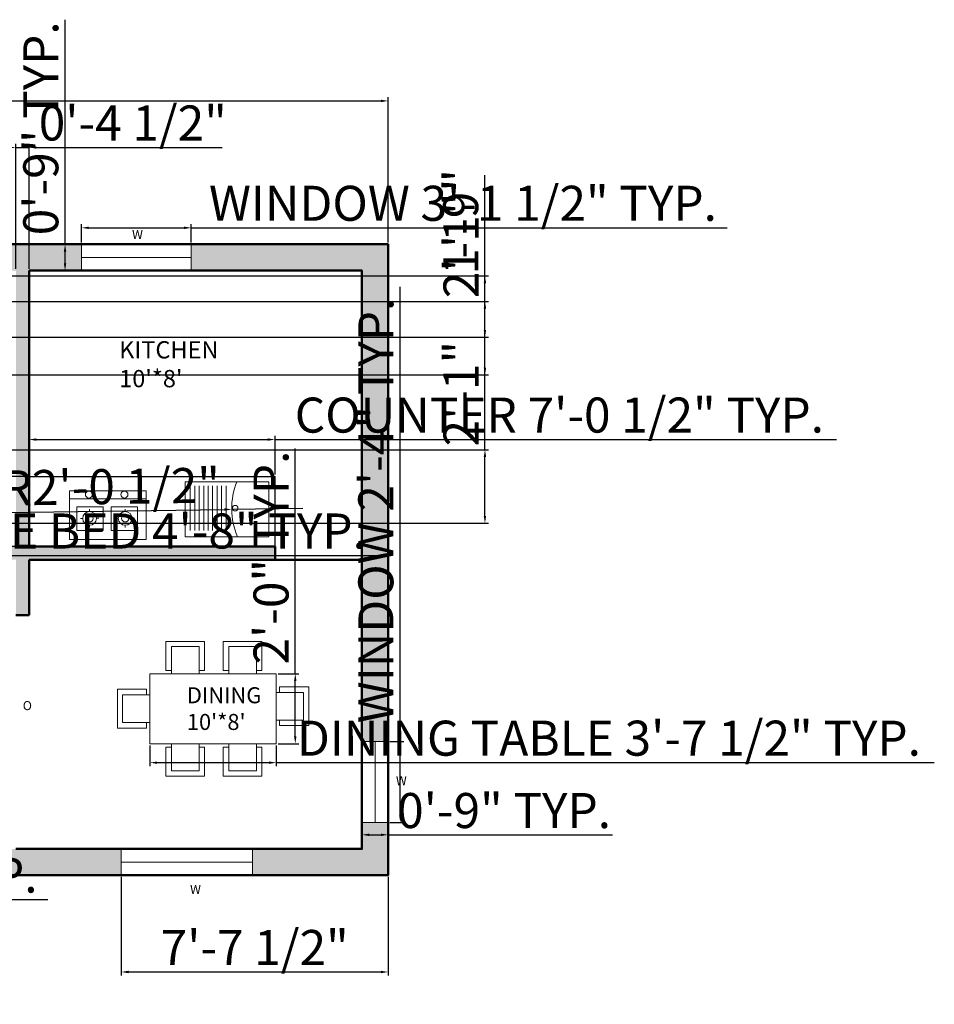
# Model space of a CAD drawing. Units: inches. Extents: x 2225 to 3094, y 1739 to 2599.
# Tile 4 of 5: x 2780 to 3094, y 1755 to 2092. Entities that reach past the tile are written whole.
import ezdxf

# ---------------------------------------------------------------- set-up
doc = ezdxf.new("R2010")
doc.units = ezdxf.units.IN
for name, color, linetype, lineweight in [('A-ANNO-DIMS', 2, 'Continuous', 18), ('A-ANNO-TEXT', 7, 'Continuous', 18), ('A-AREA-IDEN', 7, 'Continuous', 18), ('A-EQPM', 8, 'Continuous', 18), ('A-FLOR-CASE', 9, 'Continuous', 25), ('A-FLOR-FIXT', 9, 'Continuous', 18), ('A-FURN', 8, 'Continuous', 18), ('A-WALL-PATT', 160, 'Continuous', 13), ('WALL', 7, 'Continuous', 50), ('WINDOW', 130, 'Continuous', 18)]:
    doc.layers.add(name, color=color, linetype=linetype, lineweight=lineweight)
doc.styles.get("Standard").update_dxf_attribs({"font": 'arial.ttf'})
doc.dimstyles.new('ISO-25', dxfattribs={"dimtxt": 12, "dimasz": 2.5, "dimexe": 1.25, "dimexo": 0.625, "dimtad": 1, "dimdec": 0, "dimlunit": 4, "dimtxsty": 'Standard', "dimcen": 2.5, "dimadec": 0, "dimazin": 0, "dimtfac": 1, "dimtdec": 0, "dimtmove": 0, "dimatfit": 3, "dimfxl": 1, "dimarcsym": 0})

# ---------------------------------------------------------------- blocks, each defined once
blk = doc.blocks.new('*D7')
at = {"layer": 'A-ANNO-DIMS', "color": 0, "lineweight": -2, "transparency": 16777216}
for p, q in [((2282.56, 2016.04), (2282.56, 2065.75)), ((2285.06, 2064.5), (2904.06, 2064.5)), ((2906.56, 2016.04), (2906.56, 2065.75))]:
    blk.add_line(p, q, dxfattribs=at)
at = {"layer": 'A-ANNO-DIMS', "color": 0, "transparency": 16777216}
for points in [[(2285.06, 2064.92), (2285.06, 2064.08), (2282.56, 2064.5)], [(2904.06, 2064.92), (2904.06, 2064.08), (2906.56, 2064.5)]]:
    blk.add_solid(points, dxfattribs=at)
at = {"layer": 'Defpoints', "color": 0, "transparency": 16777216}
for p in [(2906.56, 2064.5), (2282.56, 2015.41), (2906.56, 2015.41)]:
    blk.add_point(p, dxfattribs=at)
at = {"layer": 'A-ANNO-DIMS', "color": 0, "transparency": 16777216, "insert": (2594.56, 2071.25), "char_height": 12, "attachment_point": 5}
blk.add_mtext("52'", dxfattribs=at)
blk = doc.blocks.new('CHAIR-DINING')
for p, q in [((0, 1.13), (0, 11.11)), ((0, 11.11), (13.29, 11.11)), ((13.29, 1.13), (13.29, 11.11)), ((1.95, 1.13), (0, 1.13)), ((13.29, 1.13), (11.43, 1.13))]:
    blk.add_line(p, q)
blk.add_lwpolyline([(1.95, 0), (11.43, 0), (11.43, 9.33), (1.95, 9.33)], close=True)
blk = doc.blocks.new('TABLE-DINING')
blk.add_lwpolyline([(0, 23.93), (43.3, 23.93), (43.3, 0), (0, 0)], close=True)
blk = doc.blocks.new('COOKTOP-TWO-BURNER')
for p, q in [((0, 13.93), (26.27, 13.93)), ((6.81, 9.56), (6.81, 10.38)), ((19.02, 9.56), (19.02, 10.38)), ((4.52, 7.14), (3.73, 7.14)), ((9.26, 7.23), (10.04, 7.23)), ((16.73, 7.14), (15.94, 7.14)), ((21.47, 7.23), (22.24, 7.23)), ((6.9, 4.82), (6.9, 4.11)), ((19.11, 4.82), (19.11, 4.11))]:
    blk.add_line(p, q)
for points in [[(0, 0), (26.27, 0), (26.27, 16.66), (0, 16.66)], [(2.47, 11.19), (11.48, 11.19), (11.48, 3.09), (2.47, 3.09)], [(14.27, 11.19), (23.28, 11.19), (23.28, 3.09), (14.27, 3.09)]]:
    blk.add_lwpolyline(points, close=True)
for centre, radius in [((6.64, 15.37), 1.2), ((18.83, 15.37), 1.2), ((6.89, 7.19), 2.37), ((6.89, 7.19), 1.23), ((19.1, 7.19), 2.37), ((19.1, 7.19), 1.23)]:
    blk.add_circle(centre, radius)
blk = doc.blocks.new('SINK-DRAINBOARD')
for p, q in [((1.79, 17.4), (1.79, 2.15)), ((3.32, 17.4), (3.32, 2.15)), ((4.85, 17.4), (4.85, 2.15)), ((6.38, 17.4), (6.38, 2.15)), ((7.91, 17.4), (7.91, 2.15)), ((9.44, 17.4), (9.44, 2.15)), ((10.98, 17.4), (10.98, 2.15)), ((12.51, 17.4), (12.51, 2.15)), ((14.04, 17.4), (14.04, 2.15))]:
    blk.add_line(p, q)
blk.add_lwpolyline([(0, 0), (28.72, 0), (28.72, 18.77), (0, 18.77)], close=True)
blk.add_circle((17.16, 9.78), 0.951)
blk.add_arc((40.38, 9.7), 24.39, 158.1829, 203.4296)
blk = doc.blocks.new('WIN-37P6IN')
blk.add_line((0, 4.5), (37.6, 4.5))
blk.add_lwpolyline([(37.6, 0), (0, 0), (0, 9), (37.6, 9)], close=True)
blk = doc.blocks.new('WIN-44P9IN')
blk.add_line((0, 4.5), (44.94, 4.5))
blk.add_lwpolyline([(0, 0), (44.94, 0), (44.94, 9), (0, 9)], close=True)
blk = doc.blocks.new('WIN-27P8IN')
blk.add_line((4.5, 0), (4.5, 27.82))
blk.add_lwpolyline([(0, 0), (9, 0), (9, 27.82), (0, 27.82)], close=True)
blk = doc.blocks.new('KITCHEN-COUNTER-RUN')
for p, q in [((0, 0), (0, 24)), ((0, 24), (84.25, 24)), ((84.25, 0), (84.25, 24))]:
    blk.add_line(p, q)
blk = doc.blocks.new('*D26')
at = {"layer": 'A-ANNO-DIMS', "color": 0, "lineweight": -2, "transparency": 16777216}
for p, q in [((2666.23, 1916.66), (2666.23, 1907.61)), ((2722.41, 1916.66), (2722.41, 1907.61)), ((2668.73, 1908.86), (2719.91, 1908.86)), ((2722.41, 1908.86), (2904.52, 1908.86))]:
    blk.add_line(p, q, dxfattribs=at)
at = {"layer": 'A-ANNO-DIMS', "color": 0, "transparency": 16777216}
for points in [[(2668.73, 1909.27), (2668.73, 1908.44), (2666.23, 1908.86)], [(2719.91, 1909.27), (2719.91, 1908.44), (2722.41, 1908.86)]]:
    blk.add_solid(points, dxfattribs=at)
at = {"layer": 'Defpoints', "color": 0, "transparency": 16777216}
for p in [(2666.23, 1917.28), (2722.41, 1917.28), (2722.41, 1908.86)]:
    blk.add_point(p, dxfattribs=at)
at = {"layer": 'A-ANNO-DIMS', "color": 0, "transparency": 16777216, "insert": (2814.71, 1915.69), "char_height": 12, "attachment_point": 5}
blk.add_mtext('SINGLE BED 4\'-8" TYP.', dxfattribs=at)
blk = doc.blocks.new('*D30')
at = {"layer": 'A-ANNO-DIMS', "color": 0, "lineweight": -2, "transparency": 16777216}
for p, q in [((2824.95, 1843.8), (2824.95, 1836.68)), ((2868.25, 1843.8), (2868.25, 1836.68)), ((2827.45, 1837.93), (2865.75, 1837.93)), ((2868.25, 1837.93), (3093.61, 1837.93))]:
    blk.add_line(p, q, dxfattribs=at)
at = {"layer": 'A-ANNO-DIMS', "color": 0, "transparency": 16777216}
for points in [[(2827.45, 1838.34), (2827.45, 1837.51), (2824.95, 1837.93)], [(2865.75, 1838.34), (2865.75, 1837.51), (2868.25, 1837.93)]]:
    blk.add_solid(points, dxfattribs=at)
at = {"layer": 'Defpoints', "color": 0, "transparency": 16777216}
for p in [(2824.95, 1844.42), (2868.25, 1844.42), (2868.25, 1837.93)]:
    blk.add_point(p, dxfattribs=at)
at = {"layer": 'A-ANNO-DIMS', "color": 0, "transparency": 16777216, "insert": (2982.18, 1844.76), "char_height": 12, "attachment_point": 5}
blk.add_mtext('DINING TABLE 3\'-7 1/2" TYP.', dxfattribs=at)
blk = doc.blocks.new('*D31')
at = {"layer": 'A-ANNO-DIMS', "color": 0, "lineweight": -2, "transparency": 16777216}
for p, q in [((2874.75, 1868.35), (2874.75, 1945.46)), ((2868.88, 1868.35), (2876, 1868.35)), ((2874.75, 1846.92), (2874.75, 1865.85)), ((2868.88, 1844.42), (2876, 1844.42))]:
    blk.add_line(p, q, dxfattribs=at)
at = {"layer": 'A-ANNO-DIMS', "color": 0, "transparency": 16777216}
for points in [[(2874.33, 1865.85), (2875.17, 1865.85), (2874.75, 1868.35)], [(2874.33, 1846.92), (2875.17, 1846.92), (2874.75, 1844.42)]]:
    blk.add_solid(points, dxfattribs=at)
at = {"layer": 'Defpoints', "color": 0, "transparency": 16777216}
for p in [(2868.25, 1868.35), (2874.75, 1868.35), (2868.25, 1844.42)]:
    blk.add_point(p, dxfattribs=at)
at = {"layer": 'A-ANNO-DIMS', "color": 0, "transparency": 16777216, "insert": (2868, 1908.15), "char_height": 12, "attachment_point": 5, "rotation": 90}
blk.add_mtext('2\'-0" TYP.', dxfattribs=at)
blk = doc.blocks.new('*D42')
at = {"layer": 'A-ANNO-DIMS', "color": 0, "lineweight": -2, "transparency": 16777216}
for p, q in [((2783.56, 1936.54), (2783.56, 1949.8)), ((2786.06, 1948.55), (2865.31, 1948.55)), ((2867.81, 1936.54), (2867.81, 1949.8)), ((2867.81, 1948.55), (3060.07, 1948.55))]:
    blk.add_line(p, q, dxfattribs=at)
at = {"layer": 'A-ANNO-DIMS', "color": 0, "transparency": 16777216}
for points in [[(2786.06, 1948.97), (2786.06, 1948.13), (2783.56, 1948.55)], [(2865.31, 1948.97), (2865.31, 1948.13), (2867.81, 1948.55)]]:
    blk.add_solid(points, dxfattribs=at)
at = {"layer": 'Defpoints', "color": 0, "transparency": 16777216}
for p in [(2867.81, 1948.55), (2783.56, 1935.91), (2867.81, 1935.91)]:
    blk.add_point(p, dxfattribs=at)
at = {"layer": 'A-ANNO-DIMS', "color": 0, "transparency": 16777216, "insert": (2965.19, 1955.38), "char_height": 12, "attachment_point": 5}
blk.add_mtext('COUNTER 7\'-0 1/2" TYP.', dxfattribs=at)
blk = doc.blocks.new('*D43')
at = {"layer": 'A-ANNO-DIMS', "color": 0, "lineweight": -2, "transparency": 16777216}
for p, q in [((2770.92, 1935.91), (2770.92, 2013.01)), ((2782.93, 1935.91), (2769.67, 1935.91)), ((2770.92, 1914.41), (2770.92, 1933.41)), ((2782.93, 1911.91), (2769.67, 1911.91))]:
    blk.add_line(p, q, dxfattribs=at)
at = {"layer": 'A-ANNO-DIMS', "color": 0, "transparency": 16777216}
for points in [[(2770.5, 1933.41), (2771.34, 1933.41), (2770.92, 1935.91)], [(2770.5, 1914.41), (2771.34, 1914.41), (2770.92, 1911.91)]]:
    blk.add_solid(points, dxfattribs=at)
at = {"layer": 'Defpoints', "color": 0, "transparency": 16777216}
for p in [(2770.92, 1935.91), (2783.56, 1935.91), (2783.56, 1911.91)]:
    blk.add_point(p, dxfattribs=at)
at = {"layer": 'A-ANNO-DIMS', "color": 0, "transparency": 16777216, "insert": (2764.17, 1975.71), "char_height": 12, "attachment_point": 5, "rotation": 90}
blk.add_mtext('2\'-0" TYP.', dxfattribs=at)
blk = doc.blocks.new('*D46')
at = {"layer": 'A-ANNO-DIMS', "color": 0, "lineweight": -2, "transparency": 16777216}
for p, q in [((2801.54, 2016.04), (2801.54, 2022.3)), ((2804.04, 2021.05), (2836.64, 2021.05)), ((2839.14, 2016.04), (2839.14, 2022.3)), ((2839.14, 2021.05), (3022.7, 2021.05))]:
    blk.add_line(p, q, dxfattribs=at)
at = {"layer": 'A-ANNO-DIMS', "color": 0, "transparency": 16777216}
for points in [[(2804.04, 2021.47), (2804.04, 2020.63), (2801.54, 2021.05)], [(2836.64, 2021.47), (2836.64, 2020.63), (2839.14, 2021.05)]]:
    blk.add_solid(points, dxfattribs=at)
at = {"layer": 'Defpoints', "color": 0, "transparency": 16777216}
for p in [(2839.14, 2021.05), (2801.54, 2015.41), (2839.14, 2015.41)]:
    blk.add_point(p, dxfattribs=at)
at = {"layer": 'A-ANNO-DIMS', "color": 0, "transparency": 16777216, "insert": (2932.17, 2027.89), "char_height": 12, "attachment_point": 5}
blk.add_mtext('WINDOW 3\'-1 1/2" TYP.', dxfattribs=at)
blk = doc.blocks.new('*D47')
at = {"layer": 'A-ANNO-DIMS', "color": 0, "lineweight": -2, "transparency": 16777216}
for p, q in [((2795.9, 2015.41), (2795.9, 2092.31)), ((2800.91, 2015.41), (2794.65, 2015.41)), ((2795.9, 2008.91), (2795.9, 2012.91)), ((2800.91, 2006.41), (2794.65, 2006.41))]:
    blk.add_line(p, q, dxfattribs=at)
at = {"layer": 'A-ANNO-DIMS', "color": 0, "transparency": 16777216}
for points in [[(2795.48, 2012.91), (2796.32, 2012.91), (2795.9, 2015.41)], [(2795.48, 2008.91), (2796.32, 2008.91), (2795.9, 2006.41)]]:
    blk.add_solid(points, dxfattribs=at)
at = {"layer": 'Defpoints', "color": 0, "transparency": 16777216}
for p in [(2795.9, 2015.41), (2801.54, 2015.41), (2801.54, 2006.41)]:
    blk.add_point(p, dxfattribs=at)
at = {"layer": 'A-ANNO-DIMS', "color": 0, "transparency": 16777216, "insert": (2789.15, 2055.11), "char_height": 12, "attachment_point": 5, "rotation": 90}
blk.add_mtext('0\'-9" TYP.', dxfattribs=at)
blk = doc.blocks.new('*D50')
at = {"layer": 'A-ANNO-DIMS', "color": 0, "lineweight": -2, "transparency": 16777216}
for p, q in [((2910.73, 1845.22), (2910.73, 2000.82)), ((2907.18, 1845.22), (2911.98, 1845.22)), ((2910.73, 1819.9), (2910.73, 1842.72)), ((2907.18, 1817.4), (2911.98, 1817.4))]:
    blk.add_line(p, q, dxfattribs=at)
at = {"layer": 'A-ANNO-DIMS', "color": 0, "transparency": 16777216}
for points in [[(2910.31, 1842.72), (2911.15, 1842.72), (2910.73, 1845.22)], [(2910.31, 1819.9), (2911.15, 1819.9), (2910.73, 1817.4)]]:
    blk.add_solid(points, dxfattribs=at)
at = {"layer": 'Defpoints', "color": 0, "transparency": 16777216}
for p in [(2906.56, 1845.22), (2910.73, 1845.22), (2906.56, 1817.4)]:
    blk.add_point(p, dxfattribs=at)
at = {"layer": 'A-ANNO-DIMS', "color": 0, "transparency": 16777216, "insert": (2903.9, 1924.27), "char_height": 12, "attachment_point": 5, "rotation": 90}
blk.add_mtext('WINDOW 2\'-4" TYP.', dxfattribs=at)
blk = doc.blocks.new('*D51')
at = {"layer": 'A-ANNO-DIMS', "color": 0, "lineweight": -2, "transparency": 16777216}
for p, q in [((2897.56, 1816.77), (2897.56, 1811.98)), ((2906.56, 1816.77), (2906.56, 1811.98)), ((2900.06, 1813.23), (2904.06, 1813.23)), ((2906.56, 1813.23), (2983.45, 1813.23))]:
    blk.add_line(p, q, dxfattribs=at)
at = {"layer": 'A-ANNO-DIMS', "color": 0, "transparency": 16777216}
for points in [[(2900.06, 1813.64), (2900.06, 1812.81), (2897.56, 1813.23)], [(2904.06, 1813.64), (2904.06, 1812.81), (2906.56, 1813.23)]]:
    blk.add_solid(points, dxfattribs=at)
at = {"layer": 'Defpoints', "color": 0, "transparency": 16777216}
for p in [(2897.56, 1817.4), (2906.56, 1817.4), (2906.56, 1813.23)]:
    blk.add_point(p, dxfattribs=at)
at = {"layer": 'A-ANNO-DIMS', "color": 0, "transparency": 16777216, "insert": (2946.26, 1819.98), "char_height": 12, "attachment_point": 5}
blk.add_mtext('0\'-9" TYP.', dxfattribs=at)
blk = doc.blocks.new('*D52')
at = {"layer": 'A-ANNO-DIMS', "color": 0, "lineweight": -2, "transparency": 16777216}
for p, q in [((2550.8, 1798.79), (2550.8, 1789.81)), ((2606.48, 1798.79), (2606.48, 1789.81)), ((2553.3, 1791.06), (2603.98, 1791.06)), ((2606.48, 1791.06), (2790.04, 1791.06))]:
    blk.add_line(p, q, dxfattribs=at)
at = {"layer": 'A-ANNO-DIMS', "color": 0, "transparency": 16777216}
for points in [[(2553.3, 1791.48), (2553.3, 1790.64), (2550.8, 1791.06)], [(2603.98, 1791.48), (2603.98, 1790.64), (2606.48, 1791.06)]]:
    blk.add_solid(points, dxfattribs=at)
at = {"layer": 'Defpoints', "color": 0, "transparency": 16777216}
for p in [(2550.8, 1799.41), (2606.48, 1799.41), (2606.48, 1791.06)]:
    blk.add_point(p, dxfattribs=at)
at = {"layer": 'A-ANNO-DIMS', "color": 0, "transparency": 16777216, "insert": (2699.51, 1797.89), "char_height": 12, "attachment_point": 5}
blk.add_mtext('WINDOW 4\'-7 1/2" TYP.', dxfattribs=at)
blk = doc.blocks.new('*D67')
at = {"layer": 'A-ANNO-DIMS', "color": 0, "lineweight": -2, "transparency": 16777216}
for p, q in [((2815.14, 1798.79), (2815.14, 1765.01)), ((2906.56, 1798.79), (2906.56, 1765.01)), ((2817.64, 1766.26), (2904.06, 1766.26))]:
    blk.add_line(p, q, dxfattribs=at)
at = {"layer": 'A-ANNO-DIMS', "color": 0, "transparency": 16777216}
for points in [[(2817.64, 1766.68), (2817.64, 1765.84), (2815.14, 1766.26)], [(2904.06, 1766.68), (2904.06, 1765.84), (2906.56, 1766.26)]]:
    blk.add_solid(points, dxfattribs=at)
at = {"layer": 'Defpoints', "color": 0, "transparency": 16777216}
for p in [(2815.14, 1799.41), (2906.56, 1799.41), (2906.56, 1766.26)]:
    blk.add_point(p, dxfattribs=at)
at = {"layer": 'A-ANNO-DIMS', "color": 0, "transparency": 16777216, "insert": (2860.85, 1773.09), "char_height": 12, "attachment_point": 5}
blk.add_mtext('7\'-7 1/2"', dxfattribs=at)
blk = doc.blocks.new('*D71')
at = {"layer": 'A-ANNO-DIMS', "color": 0, "lineweight": -2, "transparency": 16777216}
for p, q in [((2939.71, 1995.85), (2939.71, 2031.7)), ((2500.68, 1995.85), (2940.96, 1995.85)), ((2939.71, 1973.17), (2939.71, 1993.35)), ((2499.96, 1970.67), (2940.96, 1970.67))]:
    blk.add_line(p, q, dxfattribs=at)
at = {"layer": 'A-ANNO-DIMS', "color": 0, "transparency": 16777216}
for points in [[(2939.29, 1993.35), (2940.12, 1993.35), (2939.71, 1995.85)], [(2939.29, 1973.17), (2940.12, 1973.17), (2939.71, 1970.67)]]:
    blk.add_solid(points, dxfattribs=at)
at = {"layer": 'Defpoints', "color": 0, "transparency": 16777216}
for p in [(2500.06, 1995.85), (2939.71, 1995.85), (2499.34, 1970.67)]:
    blk.add_point(p, dxfattribs=at)
at = {"layer": 'A-ANNO-DIMS', "color": 0, "transparency": 16777216, "insert": (2933.06, 2015.03), "char_height": 12, "attachment_point": 5, "rotation": 90}
blk.add_mtext('2\'-1"', dxfattribs=at)
blk = doc.blocks.new('*D73')
at = {"layer": 'A-ANNO-DIMS', "color": 0, "lineweight": -2, "transparency": 16777216}
for p, q in [((2939.71, 1945.09), (2939.71, 1980.94)), ((2535.18, 1945.09), (2940.96, 1945.09)), ((2939.71, 1922.41), (2939.71, 1942.59)), ((2534.46, 1919.91), (2940.96, 1919.91))]:
    blk.add_line(p, q, dxfattribs=at)
at = {"layer": 'A-ANNO-DIMS', "color": 0, "transparency": 16777216}
for points in [[(2939.29, 1942.59), (2940.12, 1942.59), (2939.71, 1945.09)], [(2939.29, 1922.41), (2940.12, 1922.41), (2939.71, 1919.91)]]:
    blk.add_solid(points, dxfattribs=at)
at = {"layer": 'Defpoints', "color": 0, "transparency": 16777216}
for p in [(2534.56, 1945.09), (2939.71, 1945.09), (2533.84, 1919.91)]:
    blk.add_point(p, dxfattribs=at)
at = {"layer": 'A-ANNO-DIMS', "color": 0, "transparency": 16777216, "insert": (2933.06, 1964.27), "char_height": 12, "attachment_point": 5, "rotation": 90}
blk.add_mtext('2\'-1"', dxfattribs=at)
blk = doc.blocks.new('*D77')
at = {"layer": 'A-ANNO-DIMS', "color": 0, "lineweight": -2, "transparency": 16777216}
for p, q in [((2939.71, 2004.59), (2939.71, 2039.11)), ((2591.98, 2004.59), (2940.96, 2004.59)), ((2939.71, 1986.09), (2939.71, 2002.09)), ((2591.98, 1983.59), (2940.96, 1983.59))]:
    blk.add_line(p, q, dxfattribs=at)
at = {"layer": 'A-ANNO-DIMS', "color": 0, "transparency": 16777216}
for points in [[(2939.29, 2002.09), (2940.12, 2002.09), (2939.71, 2004.59)], [(2939.29, 1986.09), (2940.12, 1986.09), (2939.71, 1983.59)]]:
    blk.add_solid(points, dxfattribs=at)
at = {"layer": 'Defpoints', "color": 0, "transparency": 16777216}
for p in [(2591.35, 2004.59), (2939.71, 2004.59), (2591.35, 1983.59)]:
    blk.add_point(p, dxfattribs=at)
at = {"layer": 'A-ANNO-DIMS', "color": 0, "transparency": 16777216, "insert": (2932.96, 2023.1), "char_height": 12, "attachment_point": 5, "rotation": 90}
blk.add_mtext('1\'-9"', dxfattribs=at)
blk = doc.blocks.new('*D78')
at = {"layer": 'A-ANNO-DIMS', "color": 0, "lineweight": -2, "transparency": 16777216}
for p, q in [((2779.06, 2007.04), (2779.06, 2049.81)), ((2783.56, 2007.04), (2783.56, 2049.81)), ((2776.56, 2048.56), (2774.06, 2048.56)), ((2779.06, 2048.56), (2783.56, 2048.56)), ((2786.06, 2048.56), (2849.67, 2048.56))]:
    blk.add_line(p, q, dxfattribs=at)
at = {"layer": 'A-ANNO-DIMS', "color": 0, "transparency": 16777216}
for points in [[(2776.56, 2048.98), (2776.56, 2048.14), (2779.06, 2048.56)], [(2786.06, 2048.98), (2786.06, 2048.14), (2783.56, 2048.56)]]:
    blk.add_solid(points, dxfattribs=at)
at = {"layer": 'Defpoints', "color": 0, "transparency": 16777216}
for p in [(2783.56, 2048.56), (2779.06, 2006.41), (2783.56, 2006.41)]:
    blk.add_point(p, dxfattribs=at)
at = {"layer": 'A-ANNO-DIMS', "color": 0, "transparency": 16777216, "insert": (2819.11, 2055.39), "char_height": 12, "attachment_point": 5}
blk.add_mtext('0\'-4 1/2"', dxfattribs=at)
blk = doc.blocks.new('*D79')
at = {"layer": 'A-ANNO-DIMS', "color": 0, "lineweight": -2, "transparency": 16777216}
for p, q in [((2877.38, 1924.99), (2852.99, 1924.65)), ((2775.41, 1923.56), (2850.49, 1924.61))]:
    blk.add_line(p, q, dxfattribs=at)
at = {"layer": 'A-ANNO-DIMS', "color": 0, "transparency": 16777216}
blk.add_solid([(2850.49, 1925.03), (2850.5, 1924.2), (2852.99, 1924.65)], dxfattribs=at)
at = {"layer": 'Defpoints', "color": 0, "transparency": 16777216}
for p in [(2877.38, 1924.99), (2852.99, 1924.65)]:
    blk.add_point(p, dxfattribs=at)
at = {"layer": 'A-ANNO-DIMS', "color": 0, "transparency": 16777216, "insert": (2811.6, 1930.9), "char_height": 12, "attachment_point": 5, "rotation": 0.8061}
blk.add_mtext('R2\'-0 1/2"', dxfattribs=at)

msp = doc.modelspace()

# ---------------------------------------------------------------- hatches: boundary and pattern name
at = {"layer": 'A-WALL-PATT'}
h = msp.add_hatch(color=256, dxfattribs=at)
h.dxf.hatch_style = 1
h.paths.add_polyline_path([(2445.16, 2015.41), (2282.56, 2015.41), (2282.56, 1948.06), (2291.56, 1948.06), (2291.56, 2006.41), (2445.16, 2006.41)], flags=17)
h.paths.add_polyline_path([(2528.69, 2015.41), (2482.76, 2015.41), (2482.76, 2006.41), (2495.56, 2006.41), (2495.56, 1995.86), (2499.34, 1995.86, -0.007163), (2500.06, 1995.85), (2500.06, 2006.41), (2528.69, 2006.41)], flags=17)
h.paths.add_polyline_path([(2867.81, 1911.91), (2783.56, 1911.91), (2783.56, 1935.91), (2783.56, 2006.41), (2801.54, 2006.41), (2801.54, 2015.41), (2758.39, 2015.41), (2758.39, 2006.41), (2779.06, 2006.41), (2779.06, 1911.91), (2767.43, 1911.91), (2767.43, 1907.41), (2779.06, 1907.41), (2779.06, 1888.45), (2783.56, 1888.45), (2783.56, 1907.41), (2867.81, 1907.41)])
h.paths.add_polyline_path([(2906.56, 2015.41), (2839.14, 2015.41), (2839.14, 2006.41), (2897.56, 2006.41), (2897.56, 1911.91), (2897.56, 1907.41), (2897.56, 1845.22), (2906.56, 1845.22)])
h.paths.add_polyline_path([(2906.56, 1817.4), (2897.56, 1817.4), (2897.56, 1808.41), (2860.08, 1808.41), (2860.08, 1799.41), (2906.56, 1799.41)])
h.paths.add_polyline_path([(2815.14, 1808.41), (2783.56, 1808.41), (2779.06, 1808.41), (2727.64, 1808.41), (2606.48, 1808.41), (2606.48, 1799.41), (2815.14, 1799.41)])
h.paths.add_polyline_path([(2780.45, 1854.18), (2785.35, 1854.18), (2785.35, 1860.55), (2780.45, 1860.55)], flags=9)
h.paths.add_polyline_path([(2500.16, 1831.65), (2508.42, 1831.65), (2508.42, 1838.02), (2500.16, 1838.02)], flags=25)
h.paths.add_polyline_path([(2745.49, 1907.67), (2750.15, 1907.67), (2750.15, 1914.04), (2745.49, 1914.04)], flags=9)
h.paths.add_polyline_path([(2651.86, 1972.18), (2656.53, 1972.18), (2656.53, 1978.54), (2651.86, 1978.54)], flags=9)
h.paths.add_polyline_path([(2493.47, 1911.25), (2498.13, 1911.25), (2498.13, 1917.61), (2493.47, 1917.61)], flags=25)
h.paths.add_polyline_path([(2530.27, 1929.7), (2534.93, 1929.7), (2534.93, 1936.07), (2530.27, 1936.07)], flags=25)
h.paths.add_polyline_path([(2432.89, 1863.65), (2450.26, 1863.65), (2450.26, 1875.18), (2432.89, 1875.18)], flags=25)
h.paths.add_polyline_path([(2735.79, 1821.76), (2748.37, 1821.76), (2748.37, 1828.13), (2735.79, 1828.13)], flags=9)
h.paths.add_polyline_path([(2717.02, 1870.02), (2747.35, 1870.02), (2747.35, 1881.55), (2717.02, 1881.55)], flags=9)
h.paths.add_polyline_path([(2839.5, 1851.69), (2856.29, 1851.69), (2856.29, 1863.22), (2839.5, 1863.22)], flags=25)
h.paths.add_polyline_path([(2825.64, 1966.59), (2846.28, 1966.59), (2846.28, 1978.12), (2825.64, 1978.12)], flags=25)
h.paths.add_polyline_path([(2692.05, 1977.43), (2722.05, 1977.43), (2722.05, 1988.96), (2692.05, 1988.96)], flags=9)
h.paths.add_polyline_path([(2282.56, 1948.06), (2291.56, 1948.06), (2291.56, 2006.41), (2445.16, 2006.41), (2445.16, 2015.41), (2282.56, 2015.41)])
h.paths.add_polyline_path([(2291.56, 1922.71), (2282.56, 1922.71), (2282.56, 1799.41), (2550.8, 1799.41), (2550.8, 1808.41), (2500.06, 1808.41), (2500.06, 1817.48), (2495.56, 1817.48), (2495.56, 1808.41), (2291.56, 1808.41), (2291.56, 1887.91), (2327.56, 1887.91), (2495.56, 1887.91), (2495.56, 1857.48), (2500.06, 1857.48), (2500.06, 1887.91), (2500.06, 1898.14), (2495.56, 1898.14), (2495.56, 1892.41), (2291.56, 1892.41)])

# ---------------------------------------------------------------- linework, layer by layer
at = {"layer": 'WALL'}
for p, q in [((2783.56, 2006.41), (2783.56, 1911.91)), ((2897.56, 1907.41), (2897.56, 1915.42)), ((2783.56, 1911.91), (2867.81, 1911.91)), ((2867.81, 1907.41), (2867.81, 1911.91)), ((2783.56, 1907.41), (2897.56, 1907.41)), ((2783.56, 1907.41), (2783.56, 1888.45)), ((2779.06, 1888.45), (2783.56, 1888.45)), ((2779.06, 1808.41), (2783.56, 1808.41)), ((2897.56, 1808.41), (2783.56, 1808.41))]:
    msp.add_line(p, q, dxfattribs=at)
msp.add_lwpolyline([(2282.56, 1799.41), (2906.56, 1799.41), (2906.56, 2015.41), (2282.56, 2015.41)], close=True, dxfattribs=at)
for points in [[(2897.56, 1911.91), (2897.56, 2006.41), (2783.56, 2006.41)], [(2783.56, 1808.41), (2897.56, 1808.41), (2897.56, 1907.41)]]:
    msp.add_lwpolyline(points, dxfattribs=at)

# ---------------------------------------------------------------- block references
at = {"layer": 'A-EQPM'}
msp.add_blockref('COOKTOP-TWO-BURNER', (2797.42, 1914.37), dxfattribs=at)
at = {"layer": 'A-FLOR-CASE'}
msp.add_blockref('KITCHEN-COUNTER-RUN', (2783.56, 1911.91), dxfattribs=at)
at = {"layer": 'A-FLOR-FIXT'}
msp.add_blockref('SINK-DRAINBOARD', (2837, 1915.29), dxfattribs=at)
at = {"layer": 'A-FURN'}
for name, p in [('CHAIR-DINING', (2830.39, 1868.35)), ('CHAIR-DINING', (2850.04, 1868.35)), ('TABLE-DINING', (2824.95, 1844.42))]:
    msp.add_blockref(name, p, dxfattribs=at)
at = {"layer": 'A-FURN', "extrusion": (0, 0, -1), "zscale": -1}
for p, rotation in [((-2824.95, 1863.08), 269.9999999999992), ((-2830.39, 1844.42), 180), ((-2850.04, 1844.42), 180)]:
    msp.add_blockref('CHAIR-DINING', p, dxfattribs=dict(at, rotation=rotation))
at = {"layer": 'A-FURN', "rotation": 269.9999999999941}
msp.add_blockref('CHAIR-DINING', (2868.25, 1863.92), dxfattribs=at)
at = {"layer": 'WINDOW'}
for name, p in [('WIN-37P6IN', (2801.54, 2006.41)), ('WIN-27P8IN', (2897.56, 1817.4)), ('WIN-44P9IN', (2815.14, 1799.41))]:
    msp.add_blockref(name, p, dxfattribs=at)

# ---------------------------------------------------------------- texts
at = {"layer": 'A-ANNO-TEXT', "char_height": 3.09, "attachment_point": 1}
for s, insert in [('W', (2818.86, 2020.27)), ('\\pxt3;O', (2781.43, 1859.01)), ('W', (2909.23, 1833.29)), ('W', (2838.73, 1796.08))]:
    msp.add_mtext_dynamic_manual_height_columns(s, width=49.525, gutter_width=15.45, heights=[0], dxfattribs=dict(at, insert=insert))
at = {"layer": 'A-AREA-IDEN', "attachment_point": 1}
for s, width, gutter_width, heights, insert, char_height in [("KITCHEN\\P10'*8'", 94.8443, 29.59, [0], (2814.43, 1982.24), 5.917), ("DINING\\P10'*8'", 87.8531, 27.41, [14.83], (2837.63, 1863.75), 5.481)]:
    msp.add_mtext_dynamic_manual_height_columns(s, width=width, gutter_width=gutter_width, heights=heights, dxfattribs=dict(at, insert=insert, char_height=char_height))

# ---------------------------------------------------------------- dimensions: what is measured, and where the dimension line sits
at = {"layer": 'A-ANNO-DIMS'}
for base, p1, p2, text, picture, middle in [((2795.9, 2015.41), (2801.54, 2006.41), (2801.54, 2015.41), '<> TYP.', '*D47', (2789.15, 2055.11)), ((2770.92, 1935.91), (2783.56, 1911.91), (2783.56, 1935.91), '<> TYP.', '*D43', (2764.17, 1975.71)), ((2910.73, 1845.22), (2906.56, 1817.4), (2906.56, 1845.22), 'WINDOW <> TYP.', '*D50', (2903.9, 1924.27)), ((2874.75, 1868.35), (2868.25, 1844.42), (2868.25, 1868.35), '<> TYP.', '*D31', (2868, 1908.15))]:
    dim = msp.add_linear_dim(base=base, p1=p1, p2=p2, angle=90, text=text, dimstyle='ISO-25', override={"dimdec": 1, "dimlfac": 1, "dimrnd": 0, "dimzin": 1, "dimdsep": 46, "dimlunit": 4, "dimfrac": 2}, dxfattribs=at)
    dim.commit()
    dim.dimension.update_dxf_attribs({"geometry": picture, "text_midpoint": middle})
for base, p1, p2, override, picture, middle in [((2906.56, 2064.5), (2282.56, 2015.41), (2906.56, 2015.41), {"dimclrd": 0, "dimclre": 0, "dimclrt": 0}, '*D7', (2594.56, 2071.25)), ((2783.56, 2048.56), (2779.06, 2006.41), (2783.56, 2006.41), {"dimdec": 1, "dimlfac": 1, "dimrnd": 0, "dimzin": 1, "dimdsep": 46, "dimlunit": 4, "dimfrac": 2}, '*D78', (2819.11, 2055.39)), ((2906.56, 1766.26), (2815.14, 1799.41), (2906.56, 1799.41), {"dimdec": 1, "dimlfac": 1, "dimrnd": 0, "dimzin": 1, "dimdsep": 46, "dimlunit": 4, "dimfrac": 2}, '*D67', (2860.85, 1773.09))]:
    dim = msp.add_linear_dim(base=base, p1=p1, p2=p2, dimstyle='ISO-25', override=override, dxfattribs=at)
    dim.commit()
    dim.dimension.update_dxf_attribs({"geometry": picture, "text_midpoint": middle})
for base, p1, p2, text, picture, middle in [((2839.14, 2021.05), (2801.54, 2015.41), (2839.14, 2015.41), 'WINDOW <> TYP.', '*D46', (2932.17, 2027.89)), ((2867.8115, 1948.5496), (2783.5575, 1935.9115), (2867.8115, 1935.9115), 'COUNTER <> TYP.', '*D42', (2965.1929, 1955.3833)), ((2722.41, 1908.86), (2666.23, 1917.28), (2722.41, 1917.28), 'SINGLE BED <> TYP.', '*D26', (2814.71, 1915.69)), ((2868.25, 1837.93), (2824.95, 1844.42), (2868.25, 1844.42), 'DINING TABLE <> TYP.', '*D30', (2982.18, 1844.76)), ((2906.56, 1813.23), (2897.56, 1817.4), (2906.56, 1817.4), '<> TYP.', '*D51', (2946.26, 1819.98)), ((2606.48, 1791.06), (2550.8, 1799.41), (2606.48, 1799.41), 'WINDOW <> TYP.', '*D52', (2699.51, 1797.89))]:
    dim = msp.add_linear_dim(base=base, p1=p1, p2=p2, text=text, dimstyle='ISO-25', override={"dimdec": 1, "dimlfac": 1, "dimrnd": 0, "dimzin": 1, "dimdsep": 46, "dimlunit": 4, "dimfrac": 2}, dxfattribs=at)
    dim.commit()
    dim.dimension.update_dxf_attribs({"geometry": picture, "text_midpoint": middle})
for base, p1, p2, picture, middle in [((2939.71, 2004.59), (2591.35, 1983.59), (2591.35, 2004.59), '*D77', (2932.96, 2023.1)), ((2939.71, 1995.85), (2499.34, 1970.67), (2500.06, 1995.85), '*D71', (2933.06, 2015.03)), ((2939.71, 1945.09), (2533.84, 1919.91), (2534.56, 1945.09), '*D73', (2933.06, 1964.27))]:
    dim = msp.add_linear_dim(base=base, p1=p1, p2=p2, angle=90, dimstyle='ISO-25', override={"dimdec": 1, "dimlfac": 1, "dimrnd": 0, "dimzin": 1, "dimdsep": 46, "dimlunit": 4, "dimfrac": 2}, dxfattribs=at)
    dim.commit()
    dim.dimension.update_dxf_attribs({"geometry": picture, "text_midpoint": middle})
dim = msp.add_radius_dim(center=(2877.38, 1924.99), mpoint=(2852.99, 1924.65), dimstyle='ISO-25', override={"dimdec": 1, "dimlfac": 1, "dimrnd": 0, "dimzin": 1, "dimdsep": 46, "dimlunit": 4, "dimfrac": 2}, dxfattribs=at)
dim.commit()
dim.dimension.update_dxf_attribs({"geometry": '*D79', "text_midpoint": (2811.6, 1930.9)})

doc.saveas('drawing.dxf')
